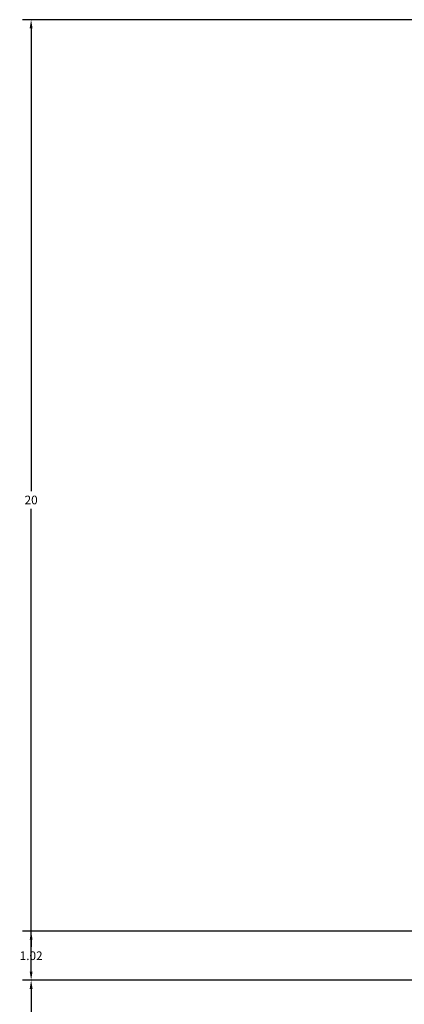
# Model space of a CAD drawing. Units: millimetres. Extents: x 446512 to 447461, y 70395 to 70610.
# Tile 10 of 39: x 446678 to 446686, y 70473 to 70493. Entities that reach past the tile are written whole.
import ezdxf

# ---------------------------------------------------------------- set-up
doc = ezdxf.new("R2010")
doc.units = ezdxf.units.MM
doc.layers.add('A-ANNO-DIMS', color=2, linetype='Continuous', lineweight=18)
doc.styles.get("Standard").update_dxf_attribs({"font": 'arial.ttf'})
doc.dimstyles.get("Standard").update_dxf_attribs({"dimtxt": 0.18, "dimasz": 0.18, "dimexe": 0.18, "dimexo": 0.0625, "dimgap": 0.09, "dimtad": 0, "dimtih": 1, "dimtoh": 1, "dimdec": 4, "dimzin": 0, "dimdsep": 46, "dimtxsty": 'Standard', "dimcen": 0.09, "dimadec": 0, "dimazin": 0, "dimtfac": 1, "dimtdec": 4, "dimtofl": 0, "dimtmove": 0, "dimatfit": 3, "dimfxl": 1, "dimtolj": 1, "dimtzin": 0, "dimarcsym": 0})

# ---------------------------------------------------------------- blocks, each defined once
blk = doc.blocks.new('*D20')
at = {"layer": 'A-ANNO-DIMS', "color": 0, "lineweight": -2, "transparency": 16777216}
for p, q in [((446686.51, 70473.382), (446678.043, 70473.382)), ((446678.223, 70473.202), (446678.223, 70463.563)), ((446678.223, 70453.562), (446678.223, 70463.2)), ((446686.51, 70453.382), (446678.043, 70453.382))]:
    blk.add_line(p, q, dxfattribs=at)
at = {"layer": 'A-ANNO-DIMS', "color": 0, "transparency": 16777216}
for points in [[(446678.193, 70473.202), (446678.253, 70473.202), (446678.223, 70473.382)], [(446678.193, 70453.562), (446678.253, 70453.562), (446678.223, 70453.382)]]:
    blk.add_solid(points, dxfattribs=at)
at = {"layer": 'Defpoints', "color": 0, "transparency": 16777216}
for p in [(446678.223, 70473.382), (446686.573, 70473.382), (446686.573, 70453.382)]:
    blk.add_point(p, dxfattribs=at)
at = {"layer": 'A-ANNO-DIMS', "color": 0, "transparency": 16777216, "insert": (446678.223, 70463.382), "char_height": 0.18, "attachment_point": 5}
blk.add_mtext('\\A1;20', dxfattribs=at)
blk = doc.blocks.new('*D21')
at = {"layer": 'A-ANNO-DIMS', "color": 0, "lineweight": -2, "transparency": 16777216}
for p, q in [((446686.51, 70493.382), (446678.043, 70493.382)), ((446678.223, 70493.202), (446678.223, 70483.563)), ((446678.223, 70473.562), (446678.223, 70483.2)), ((446686.51, 70473.382), (446678.043, 70473.382))]:
    blk.add_line(p, q, dxfattribs=at)
at = {"layer": 'A-ANNO-DIMS', "color": 0, "transparency": 16777216}
for points in [[(446678.193, 70493.202), (446678.253, 70493.202), (446678.223, 70493.382)], [(446678.193, 70473.562), (446678.253, 70473.562), (446678.223, 70473.382)]]:
    blk.add_solid(points, dxfattribs=at)
at = {"layer": 'Defpoints', "color": 0, "transparency": 16777216}
for p in [(446678.223, 70493.382), (446686.573, 70493.382), (446686.573, 70473.382)]:
    blk.add_point(p, dxfattribs=at)
at = {"layer": 'A-ANNO-DIMS', "color": 0, "transparency": 16777216, "insert": (446678.223, 70483.382), "char_height": 0.18, "attachment_point": 5}
blk.add_mtext('\\A1;20', dxfattribs=at)
blk = doc.blocks.new('*D32')
at = {"layer": 'A-ANNO-DIMS', "color": 0, "lineweight": -2, "transparency": 16777216}
for p, q in [((446730.76, 70474.405), (446678.043, 70474.405)), ((446678.223, 70474.225), (446678.223, 70474.075)), ((446678.223, 70473.562), (446678.223, 70473.711)), ((446728.946, 70473.382), (446678.043, 70473.382))]:
    blk.add_line(p, q, dxfattribs=at)
at = {"layer": 'A-ANNO-DIMS', "color": 0, "transparency": 16777216}
for points in [[(446678.193, 70474.225), (446678.253, 70474.225), (446678.223, 70474.405)], [(446678.193, 70473.562), (446678.253, 70473.562), (446678.223, 70473.382)]]:
    blk.add_solid(points, dxfattribs=at)
at = {"layer": 'Defpoints', "color": 0, "transparency": 16777216}
for p in [(446730.822, 70474.405), (446678.223, 70473.382), (446729.008, 70473.382)]:
    blk.add_point(p, dxfattribs=at)
at = {"layer": 'A-ANNO-DIMS', "color": 0, "transparency": 16777216, "insert": (446678.223, 70473.893), "char_height": 0.18, "attachment_point": 5}
blk.add_mtext('\\A1;1.02', dxfattribs=at)

msp = doc.modelspace()

# ---------------------------------------------------------------- dimensions: what is measured, and where the dimension line sits
at = {"layer": 'A-ANNO-DIMS'}
for base, p1, p2, override, picture, middle in [((446678.2228, 70493.3816), (446686.5728, 70473.3816), (446686.5728, 70493.3816), {"dimdec": 0, "dimlfac": 1, "dimrnd": 0, "dimzin": 0, "dimdsep": 46, "dimlunit": 2}, '*D21', (446678.2228, 70483.3815)), ((446678.2228, 70473.3816), (446730.8224, 70474.4047), (446729.0084, 70473.3816), {"dimdec": 2, "dimlfac": 1, "dimrnd": 0, "dimzin": 0, "dimdsep": 46, "dimlunit": 2}, '*D32', (446678.2228, 70473.8931)), ((446678.2228, 70473.3816), (446686.5728, 70453.3816), (446686.5728, 70473.3816), {"dimdec": 0, "dimlfac": 1, "dimrnd": 0, "dimzin": 0, "dimdsep": 46, "dimlunit": 2}, '*D20', (446678.2228, 70463.3815))]:
    dim = msp.add_linear_dim(base=base, p1=p1, p2=p2, angle=90, dimstyle='Standard', override=override, dxfattribs=at)
    dim.commit()
    dim.dimension.update_dxf_attribs({"geometry": picture, "text_midpoint": middle})

doc.saveas('drawing.dxf')
